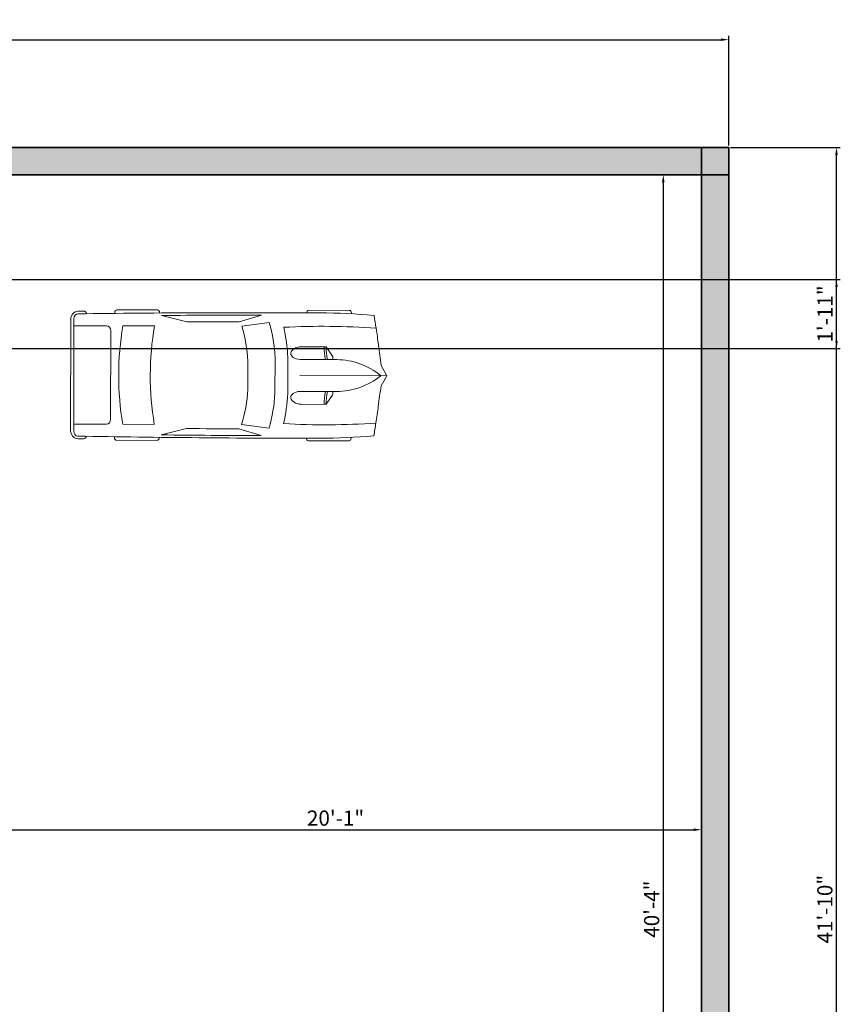
# Model space of a CAD drawing. Units: millimetres. Extents: x 2768 to 4359, y 795 to 1583.
# Tile 13 of 13: x 4089 to 4359, y 1258 to 1583. Entities that reach past the tile are written whole.
import ezdxf

# ---------------------------------------------------------------- set-up
doc = ezdxf.new("R2010")
doc.units = ezdxf.units.MM
for name, color, linetype, lineweight in [('A-ANNO-DIMS', 90, 'Continuous', 18), ('A-WALL-PATT', 140, 'Continuous', 9), ('C-PKNG-VEHI', 50, 'Continuous', 13), ('walls', 140, 'Continuous', 35)]:
    doc.layers.add(name, color=color, linetype=linetype, lineweight=lineweight)
doc.styles.get("Standard").update_dxf_attribs({"font": 'arial.ttf'})
doc.dimstyles.new('ISO-25', dxfattribs={"dimtxt": 5, "dimasz": 2.5, "dimexe": 1.25, "dimexo": 0.625, "dimtad": 1, "dimdec": 0, "dimlunit": 3, "dimtxsty": 'Standard', "dimcen": 2.5, "dimadec": 0, "dimazin": 0, "dimtfac": 1, "dimtdec": 0, "dimtmove": 0, "dimatfit": 3, "dimfxl": 1, "dimarcsym": 0})

# ---------------------------------------------------------------- blocks, each defined once
blk = doc.blocks.new('*D66')
at = {"layer": 'A-ANNO-DIMS', "color": 0, "lineweight": -2, "transparency": 16777216}
for p, q in [((4072.37, 1313.62), (4072.37, 1317.24)), ((4313.37, 1313.62), (4313.37, 1317.24)), ((4074.87, 1315.99), (4310.87, 1315.99))]:
    blk.add_line(p, q, dxfattribs=at)
at = {"layer": 'A-ANNO-DIMS', "color": 0, "transparency": 16777216}
for points in [[(4074.87, 1316.41), (4074.87, 1315.57), (4072.37, 1315.99)], [(4310.87, 1316.41), (4310.87, 1315.57), (4313.37, 1315.99)]]:
    blk.add_solid(points, dxfattribs=at)
at = {"layer": 'Defpoints', "color": 0, "transparency": 16777216}
for p in [(4313.37, 1315.99), (4072.37, 1312.99), (4313.37, 1312.99)]:
    blk.add_point(p, dxfattribs=at)
at = {"layer": 'A-ANNO-DIMS', "color": 0, "transparency": 16777216, "insert": (4192.87, 1319.17), "char_height": 5, "attachment_point": 5}
blk.add_mtext('20\'-1"', dxfattribs=at)
blk = doc.blocks.new('*D67')
at = {"layer": 'A-ANNO-DIMS', "color": 0, "lineweight": -2, "transparency": 16777216}
for p, q in [((4301.96, 1531.81), (4299.57, 1531.81)), ((4300.82, 1529.31), (4300.82, 1050.31)), ((4301.96, 1047.81), (4299.57, 1047.81))]:
    blk.add_line(p, q, dxfattribs=at)
at = {"layer": 'A-ANNO-DIMS', "color": 0, "transparency": 16777216}
for points in [[(4300.4, 1529.31), (4301.24, 1529.31), (4300.82, 1531.81)], [(4300.4, 1050.31), (4301.24, 1050.31), (4300.82, 1047.81)]]:
    blk.add_solid(points, dxfattribs=at)
at = {"layer": 'Defpoints', "color": 0, "transparency": 16777216}
for p in [(4302.59, 1531.81), (4300.82, 1047.81), (4302.59, 1047.81)]:
    blk.add_point(p, dxfattribs=at)
at = {"layer": 'A-ANNO-DIMS', "color": 0, "transparency": 16777216, "insert": (4297.64, 1289.81), "char_height": 5, "attachment_point": 5, "rotation": 90}
blk.add_mtext('40\'-4"', dxfattribs=at)
blk = doc.blocks.new('*U34')
for p, q in [((21.1, 37.41), (21.1, 36.83)), ((46.55, 38.89), (22.35, 38.89)), ((47.8, 37.39), (47.8, 37.41)), ((87.99, 31.87), (74.76, 35.92)), ((134.31, 35.6), (119.29, 31.78)), ((135.45, 37.07), (135.45, 37.41)), ((136.7, 38.89), (160.9, 38.89)), ((162.15, 37.41), (162.15, 36.77)), ((70.03, 31.54), (86.41, 29.35)), ((186.47, -33.5), (186.47, 33.5)), ((188.4, -32.76), (188.4, 32.76)), ((138.42, 29.35), (157.25, 29.35)), ((164.52, 26.39), (164.52, -26.39)), ((186.47, 29.35), (167.01, 29.35)), ((32.27, 11.63), (36.13, 17.17)), ((36.13, 17.17), (50.94, 17.17)), ((3.27, 6.13), (0.1, 0.41)), ((29.77, 9.51), (51.68, 9.51)), ((32.12, 9.51), (32.12, 11.15)), ((58.92, -10.77), (58.92, 10.77)), ((66.55, -10.53), (66.55, 10.53)), ((82.74, 8.5), (82.74, -8.5)), ((186.47, -10.53), (186.47, 10.53)), ((0, 0), (51.68, 0)), ((0.1, -0.41), (3.27, -6.13)), ((29.77, -9.51), (51.68, -9.51)), ((32.12, -9.51), (32.12, -11.15)), ((32.27, -11.63), (36.13, -17.17)), ((36.13, -17.17), (50.94, -17.17)), ((86.41, -29.35), (70.03, -31.54)), ((157.25, -29.35), (138.42, -29.35)), ((167.01, -29.35), (186.47, -29.35)), ((87.99, -31.87), (74.76, -35.92)), ((134.31, -35.6), (119.29, -31.78)), ((21.1, -37.41), (21.1, -36.83)), ((46.55, -38.89), (22.35, -38.89)), ((47.8, -37.39), (47.8, -37.41)), ((135.45, -37.07), (135.45, -37.41)), ((136.7, -38.89), (160.9, -38.89)), ((162.15, -37.41), (162.15, -36.77))]:
    blk.add_line(p, q)
for centre, major_axis, ratio, start_param, end_param in [((266.03, -27.52), (0, 313.31), 0.842304, 1.367076, 1.39176), ((41.19, -490.86), (0, 528.23), 0.842304, 0.00281, 0.075598), ((22.35, 37.41), (0, -1.48), 0.842304, 3.141593, 4.712389), ((64.48, -10555.62), (0, 10593.03), 0.842304, -0.013397, 0.002797), ((46.55, 37.41), (0, 1.48), 0.842304, -1.570796, 0), ((64.48, -10555.62), (0, -10591.55), 0.842304, 3.133765, 3.140441), ((136.7, 37.41), (0, -1.48), 0.842304, 3.141593, 4.712389), ((160.9, 37.41), (0, 1.48), 0.842304, -1.570796, 0), ((180.63, 35.84), (0, 2.22), 0.842304, -0.013017, 1.249894), ((64.48, -10556.36), (0, 10595.31), 0.842304, -0.013397, -0.013017), ((183.98, 33.5), (0, -2.96), 0.842304, 1.570796, 3.128196), ((183.98, 32.76), (0, -5.25), 0.842304, 1.570796, 3.128196), ((37.47, -593.96), (0, -623.33), 0.842304, 3.096046, 3.200911), ((135.29, 5.39), (0, 81.77), 0.842304, 1.245306, 1.50788), ((95.79, -3666.35), (0, -3698.24), 0.842304, 3.134049, 3.144098), ((259.18, -27.52), (0, -305.3), 0.842304, 4.528606, 4.561838), ((134.4, 5.39), (0, -89.78), 0.842304, 4.449482, 4.652344), ((149.6, 2.8), (0, -79.58), 0.842304, 4.372215, 4.640744), ((17.08, 0), (0, 147.02), 0.842304, 4.511394, 4.913384), ((35.91, 0), (0, 147.02), 0.842304, 4.511394, 4.913384), ((167.01, 26.39), (0, 2.96), 0.842304, 0, 1.570796), ((-204.49, 52.4), (0, -250.96), 0.842304, 1.385369, 1.434372), ((13.04, 17.01), (0, 27.42), 0.842304, 4.435146, 4.718221), ((14.2, 17.01), (0, 27.42), 0.842304, 4.435146, 4.718221), ((50.79, 13.34), (6.34, -0.36), 0.603834, -1.395552, 1.581315), ((29.77, -46.66), (0, 56.17), 0.842304, 0, 0.590319), ((32.75, 11.15), (0, 0.74), 0.842304, 0.879714, 1.570796), ((0.62, 0), (0, -0.74), 0.842304, 4.131459, 5.293319), ((29.77, 46.66), (0, 56.17), 0.842304, 2.551274, 3.141593), ((-204.49, -52.4), (0, 250.96), 0.842304, -1.434372, -1.385369), ((32.75, -11.15), (0, -0.74), 0.842304, 4.712389, 5.403472), ((13.04, -17.01), (0, -27.42), 0.842304, 1.564964, 1.848039), ((14.2, -17.01), (0, -27.42), 0.842304, 1.564964, 1.848039), ((134.4, -5.39), (0, -89.78), 0.842304, -1.510751, -1.307889), ((135.29, -5.39), (0, -81.77), 0.842304, -1.50788, -1.245306), ((149.6, -2.8), (0, -79.58), 0.842304, -1.499151, -1.230623), ((259.18, 27.52), (0, 305.3), 0.842304, 1.721348, 1.754579), ((266.03, 27.52), (0, 313.31), 0.842304, 1.749832, 1.774517), ((37.47, 593.96), (0, -623.33), 0.842304, -0.059319, 0.045547), ((167.01, -26.39), (0, -2.96), 0.842304, 4.712389, 6.283185), ((95.79, 3666.35), (0, -3698.24), 0.842304, -0.002505, 0.007544), ((183.98, -33.5), (0, 2.96), 0.842304, 3.15499, 4.712389), ((183.98, -32.76), (0, -5.25), 0.842304, 0.013397, 1.570796), ((41.19, 490.86), (0, -528.23), 0.842304, -0.075598, -0.00281), ((22.35, -37.41), (0, 1.48), 0.842304, 1.570796, 3.141593), ((64.48, 10555.62), (0, 10593.03), 0.842304, 3.138796, 3.15499), ((46.55, -37.41), (0, -1.48), 0.842304, 0, 1.570796), ((64.48, 10555.62), (0, -10591.55), 0.842304, 0.001152, 0.007828), ((136.7, -37.41), (0, -1.48), 0.842304, -1.570796, 0), ((160.9, -37.41), (0, 1.48), 0.842304, 3.141593, 4.712389), ((180.63, -35.84), (0, -2.22), 0.842304, -1.249894, 0.013017), ((64.48, 10556.36), (0, 10595.31), 0.842304, 3.15461, 3.15499)]:
    blk.add_ellipse(centre, major_axis=major_axis, ratio=ratio, start_param=start_param, end_param=end_param)
at = {"extrusion": (0, 0, -1)}
blk.add_ellipse((50.79, -13.34), major_axis=(6.34, 0.36), ratio=0.603834, start_param=-1.395552, end_param=1.581315, dxfattribs=at)
blk = doc.blocks.new('*D128')
at = {"layer": 'A-ANNO-DIMS', "color": 0, "lineweight": -2, "transparency": 16777216}
for p, q in [((3619.37, 1541.43), (3619.37, 1577.56)), ((4322.37, 1541.43), (4322.37, 1577.56)), ((3621.87, 1576.31), (4319.87, 1576.31))]:
    blk.add_line(p, q, dxfattribs=at)
at = {"layer": 'A-ANNO-DIMS', "color": 0, "transparency": 16777216}
for points in [[(3621.87, 1576.72), (3621.87, 1575.89), (3619.37, 1576.31)], [(4319.87, 1576.72), (4319.87, 1575.89), (4322.37, 1576.31)]]:
    blk.add_solid(points, dxfattribs=at)
at = {"layer": 'Defpoints', "color": 0, "transparency": 16777216}
for p in [(4322.37, 1576.31), (3619.37, 1540.81), (4322.37, 1540.81)]:
    blk.add_point(p, dxfattribs=at)
at = {"layer": 'A-ANNO-DIMS', "color": 0, "transparency": 16777216, "insert": (3970.87, 1579.49), "char_height": 5, "attachment_point": 5}
blk.add_mtext('58\'-7"', dxfattribs=at)
blk = doc.blocks.new('*D130')
at = {"layer": 'A-ANNO-DIMS', "color": 0, "lineweight": -2, "transparency": 16777216}
for p, q in [((4322.99, 1540.81), (4359.12, 1540.81)), ((4357.87, 1041.31), (4357.87, 1538.31)), ((4322.99, 1038.81), (4359.12, 1038.81))]:
    blk.add_line(p, q, dxfattribs=at)
at = {"layer": 'A-ANNO-DIMS', "color": 0, "transparency": 16777216}
for points in [[(4357.45, 1538.31), (4358.28, 1538.31), (4357.87, 1540.81)], [(4357.45, 1041.31), (4358.28, 1041.31), (4357.87, 1038.81)]]:
    blk.add_solid(points, dxfattribs=at)
at = {"layer": 'Defpoints', "color": 0, "transparency": 16777216}
for p in [(4322.37, 1540.81), (4357.87, 1540.81), (4322.37, 1038.81)]:
    blk.add_point(p, dxfattribs=at)
at = {"layer": 'A-ANNO-DIMS', "color": 0, "transparency": 16777216, "insert": (4354.69, 1289.81), "char_height": 5, "attachment_point": 5, "rotation": 90}
blk.add_mtext('41\'-10"', dxfattribs=at)
blk = doc.blocks.new('*D136')
at = {"layer": 'A-ANNO-DIMS', "color": 0, "lineweight": -2, "transparency": 16777216}
for p, q in [((3919.99, 1497.31), (4359.12, 1497.31)), ((4357.87, 1477.05), (4357.87, 1494.81)), ((3919.99, 1474.55), (4359.12, 1474.55))]:
    blk.add_line(p, q, dxfattribs=at)
at = {"layer": 'A-ANNO-DIMS', "color": 0, "transparency": 16777216}
for points in [[(4357.45, 1494.81), (4358.28, 1494.81), (4357.87, 1497.31)], [(4357.45, 1477.05), (4358.28, 1477.05), (4357.87, 1474.55)]]:
    blk.add_solid(points, dxfattribs=at)
at = {"layer": 'Defpoints', "color": 0, "transparency": 16777216}
for p in [(3919.37, 1497.31), (4357.87, 1497.31), (3919.37, 1474.55)]:
    blk.add_point(p, dxfattribs=at)
at = {"layer": 'A-ANNO-DIMS', "color": 0, "transparency": 16777216, "insert": (4354.73, 1485.93), "char_height": 5, "attachment_point": 5, "rotation": 90}
blk.add_mtext('1\'-11"', dxfattribs=at)

msp = doc.modelspace()

# ---------------------------------------------------------------- hatches: boundary and pattern name
at = {"layer": 'A-WALL-PATT'}
h = msp.add_hatch(color=256, dxfattribs=at)
h.dxf.hatch_style = 1
h.paths.add_polyline_path([(4313.37, 1540.81), (4072.37, 1540.81), (4072.37, 1531.81), (4313.37, 1531.81)])
h.paths.add_polyline_path([(4072.37, 1540.81), (4063.37, 1540.81), (4063.37, 1531.81), (4072.37, 1531.81)])
h.paths.add_polyline_path([(4322.37, 1540.81), (4313.37, 1540.81), (4313.37, 1531.81), (4322.37, 1531.81)])
h.paths.add_polyline_path([(4322.37, 1531.81), (4313.37, 1531.81), (4313.37, 1378.81), (4313.37, 1047.81), (4322.37, 1047.81), (4322.37, 1378.81)])
h.paths.add_polyline_path([(4313.37, 1047.81), (4072.37, 1047.81), (4072.37, 1038.81), (4313.37, 1038.81)])

# ---------------------------------------------------------------- linework, layer by layer
at = {"layer": 'walls'}
for p, q in [((3619.37, 1540.81), (4322.37, 1540.81)), ((4313.37, 1540.81), (4313.37, 1378.81)), ((4322.37, 1540.81), (4322.37, 1378.81)), ((3619.37, 1531.81), (4322.37, 1531.81)), ((4313.37, 1378.81), (4313.37, 1007.81)), ((4322.37, 1378.81), (4322.37, 1007.81))]:
    msp.add_line(p, q, dxfattribs=at)

# ---------------------------------------------------------------- block references
at = {"layer": 'C-PKNG-VEHI', "xscale": 0.552506122371833, "yscale": 0.552506122371833, "zscale": 0.552506122371833, "rotation": 179.8633206033408}
msp.add_blockref('*U34', (4209.71, 1465.59), dxfattribs=at)

# ---------------------------------------------------------------- dimensions: what is measured, and where the dimension line sits
at = {"layer": 'A-ANNO-DIMS'}
for base, p1, p2, override, picture, middle in [((4322.37, 1576.31), (3619.37, 1540.81), (4322.37, 1540.81), {"dimdec": 1, "dimlfac": 1, "dimrnd": 0, "dimzin": 1, "dimdsep": 46, "dimlunit": 4, "dimfrac": 2}, '*D128', (3970.87, 1579.49)), ((4313.37, 1315.99), (4072.37, 1312.99), (4313.37, 1312.99), {"dimclrd": 0, "dimclre": 0, "dimclrt": 0}, '*D66', (4192.87, 1319.17))]:
    dim = msp.add_linear_dim(base=base, p1=p1, p2=p2, dimstyle='ISO-25', override=override, dxfattribs=at)
    dim.commit()
    dim.dimension.update_dxf_attribs({"geometry": picture, "text_midpoint": middle})
for base, p1, p2, override, picture, middle in [((4357.87, 1540.81), (4322.37, 1038.81), (4322.37, 1540.81), {"dimdec": 1, "dimlfac": 1, "dimrnd": 0, "dimzin": 1, "dimdsep": 46, "dimlunit": 4, "dimfrac": 2}, '*D130', (4354.69, 1289.81)), ((4300.82, 1047.81), (4302.59, 1531.81), (4302.59, 1047.81), {"dimclrd": 0, "dimclre": 0, "dimclrt": 0}, '*D67', (4297.64, 1289.81)), ((4357.87, 1497.31), (3919.37, 1474.55), (3919.37, 1497.31), {"dimdec": 1, "dimlfac": 1, "dimrnd": 0, "dimzin": 1, "dimdsep": 46, "dimlunit": 4, "dimfrac": 2}, '*D136', (4354.73, 1485.93))]:
    dim = msp.add_linear_dim(base=base, p1=p1, p2=p2, angle=90, dimstyle='ISO-25', override=override, dxfattribs=at)
    dim.commit()
    dim.dimension.update_dxf_attribs({"geometry": picture, "text_midpoint": middle})

doc.saveas('drawing.dxf')
